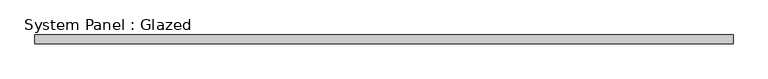
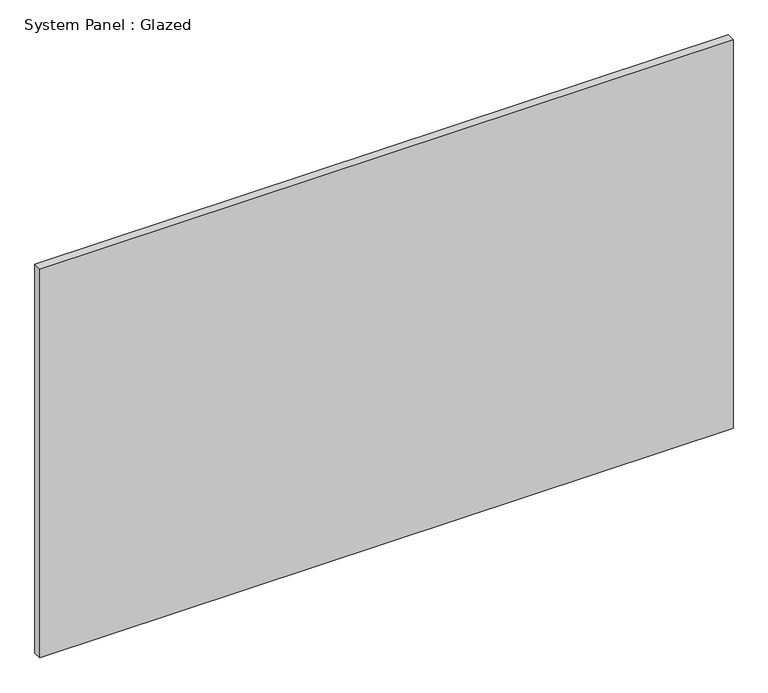
"""IFC4 building model written with IfcOpenShell, lengths in millimetres: plate geometry, System Panel : Glazed."""

from ifc_helpers import new_model, si_unit, origin, origin_with_axes, place, context, project, spatial, polyline, outline, extrude, source, transform, mapped, element, save


def system_panel_glazed_5a380d23(model_context):
    return source(origin(), model_context, "Body", "SweptSolid", [
        extrude(outline(polyline([(1028.7, 19.05), (-1028.7, 19.05), (-1028.7, 44.45), (1028.7, 44.45), (1028.7, 19.05)])), origin_with_axes(), (0.0, 0.0, 1.0), 1219.2),
    ])


if __name__ == "__main__":
    model = new_model("IFC4")
    model_context = context("Model", 3, world=origin())
    ifc_project = project(units=[si_unit("LENGTHUNIT", "METRE", prefix="MILLI")], contexts=[model_context])
    site = spatial("IfcSite", under=ifc_project)
    building = spatial("IfcBuilding", under=site)
    placement = place(None, origin())
    system_panel_glazed_shape = system_panel_glazed_5a380d23(model_context)
    element("IfcPlate", 1, ObjectType="System Panel : Glazed", at=placement, inside=building, context=model_context, shape_type="MappedRepresentation", body=[
        mapped(system_panel_glazed_shape, transform((0.0, 0.0, 0.0), x_axis=(1.0, 0.0, 0.0), y_axis=(0.0, 1.0, 0.0), z_axis=(0.0, 0.0, 1.0))),
    ])
    save(model, "model.ifc")

# Revit data of these elements
# Type "System Panel : Glazed"
#   Construction Type Id = "GSP4R"
#   Analytic Construction = "1/8 in Pilkington single glazing"
#   Visual Light Transmittance = 0.9
#   Solar Heat Gain Coefficient = 0.86
#   Heat Transfer Coefficient (U) = 1.18115 BTU/(h·ft²·°F)
# Element 1 (IfcPlate, "System Panel : Glazed")
#   Materials on its faces: "Glass"
# Materials
#   "Glass": class "Glass", colour RGB 0 128 192, transparency 0.75, Description = "Soda Lime Glass", Cost = 0
